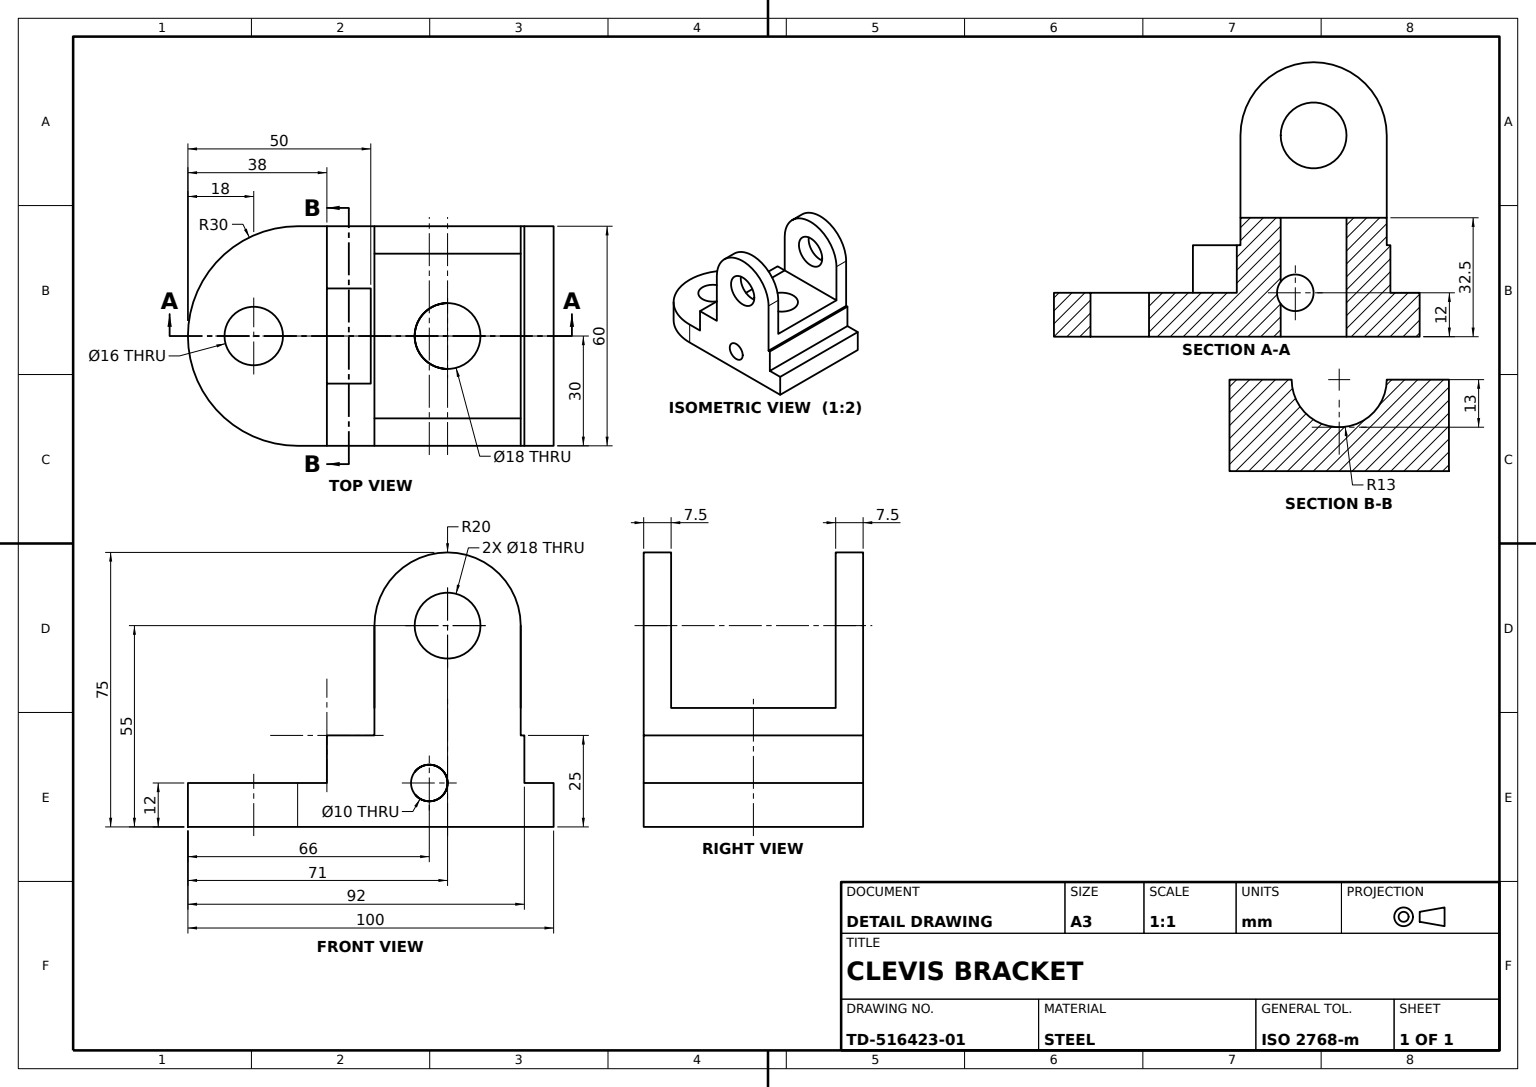
SolidWorks part; units mm, degrees
material "Plain Carbon Steel"
ref_plane "Front Plane" through (0, 0, 0) normal (0, 0, 1) x (1, 0, 0)
ref_plane "Top Plane" through (0, 0, 0) normal (0, 1, 0) x (1, 0, 0)
ref_plane "Right Plane" through (0, 0, 0) normal (1, 0, 0) x (0, 0, -1)
sketch "Base Plate Sketch" plane through (0, 0, 0) normal (0, 1, 0) x (1, 0, 0)
  line L0 (0, 0) -> (30, 0)
  line L1 (0, 0) -> (-30, 0)
  line L2 (-30, 0) -> (-30, 100)
  line L3 (-30, 100) -> (30, 100)
  line L4 (30, 100) -> (30, 0)
  dimension "D1" = 100
  dimension "D2" = 30
  dimension "D3" = 30
extrude "Base Plate" add sketch "Base Plate Sketch" along normal blind 12
sketch "Base Hole Sketch" plane through (0, 12, 0) normal (0, 1, 0) x (1, 0, 0)
  line L0 (-30, 30) -> (-30, 0)
  line L1 (-30, 0) -> (30, 0)
  line L2 (30, 0) -> (30, 30)
  circle A0 centre (0, 30) radius 30
  line M3 (-30, 0) -> (30, 0)
  line M4 (30, 0) -> (30, 100)
  line M6 (-30, 100) -> (-30, 0)
extrude "Base Hole" cut sketch "Base Hole Sketch" against normal blind 12 contours A0 M6 M3 | A0 L1 M4
sketch "Upright Block Sketch" plane through (30, 0, 0) normal (1, 0, 0) x (0, 0, -1)
  line L0 (100, 0) -> (50, 0)
  line L1 (30, 0) -> (100, 0) construction
  line L2 (50, 0) -> (50, 25)
  line L3 (50, 25) -> (62, 25)
  line L4 (62, 25) -> (92, 25)
  line L5 (92, 25) -> (92, 0)
  line L6 (30, 0) -> (30, 12) construction
  line M2 (30, 0) -> (100, 0)
  line M4 (100, 12) -> (30, 12)
  dimension "D1" = 20
  dimension "D2" = 32
  dimension "D3" = 62
  dimension "D4" = 25
extrude "Upright Block" add sketch "Upright Block Sketch" against normal blind 60 contours L5 L4 L3 L2 M4 | L5 L2 M4 M2
sketch "Clevis Ear Sketch" plane through (-30, 0, 0) normal (-1, 0, 0) x (0, 0, 1)
  line L0 (-50, 12) -> (-30, 12) construction
  line L1 (-50, 25) -> (-92, 25) construction
  line L2 (-51, 55) -> (-51, 25)
  line L3 (-51, 25) -> (-91, 25)
  line L4 (-91, 25) -> (-91, 55)
  arc A0 (-51, 55) -> (-91, 55) centre (-71, 55) ccw
  dimension "D1" = 20
  dimension "D2" = 41
  dimension "D3" = 43
extrude "Clevis Ear" add sketch "Clevis Ear Sketch" against normal blind 7.5
mirror "Clevis Ear Mirror" about plane through (0, 0, 0) normal (1, 0, 0) of "Clevis Ear"
sketch "Clevis Ear Extension Sketch" plane through (0, 25, 0) normal (0, 1, 0) x (1, 0, 0)
  line L0 (-22.5, 91) -> (-22.5, 51)
  line L1 (-22.5, 51) -> (22.5, 51)
  line L2 (22.5, 51) -> (22.5, 91)
  line L3 (22.5, 91) -> (-22.5, 91)
extrude "Clevis Ear Extension" add sketch "Clevis Ear Extension Sketch" along normal blind 7.5
sketch "Clevis Pin Bore Sketch" plane through (0, 32.5, 0) normal (0, 1, 0) x (1, 0, 0)
  line L0 (-22.5, 91) -> (-22.5, 51) construction
  line L1 (22.5, 91) -> (-22.5, 91) construction
  circle A0 centre (0, 71) radius 9
  dimension "D1" = 18
  dimension "D2" = 22.5
  dimension "D3" = 20
extrude "Clevis Pin Bore" cut sketch "Clevis Pin Bore Sketch" against normal blind 90.5
sketch "Saddle Block Sketch" plane through (30, 0, 0) normal (1, 0, 0) x (0, 0, -1)
  line L0 (50, 12) -> (38, 12)
  line L1 (30, 12) -> (50, 12) construction
  line L2 (38, 12) -> (38, 25)
  line L3 (38, 25) -> (50, 25)
  line L4 (50, 25) -> (50, 12)
  dimension "D1" = 62
extrude "Saddle Block" add sketch "Saddle Block Sketch" against normal blind 60
sketch "Saddle Cut Sketch" plane through (0, 0, -38) normal (0, 0, 1) x (1, 0, 0)
  line L0 (30, 25) -> (-30, 25) construction
  circle A0 centre (0, 25) radius 13
  dimension "D1" = 26
extrude "Saddle Cut" cut sketch "Saddle Cut Sketch" against normal blind 12
sketch "Through Hole A Sketch" plane through (-30, 0, 0) normal (-1, 0, 0) x (0, 0, 1)
  circle A0 centre (-71, 55) radius 9
  dimension "D1" = 18
extrude "Through Hole A" cut sketch "Through Hole A Sketch" against normal blind 139
sketch "Through Hole B Sketch" plane through (-30, 0, 0) normal (-1, 0, 0) x (0, 0, 1)
  circle A0 centre (-66, 12) radius 5
  dimension "D1" = 10
  dimension "D2" = 66
  dimension "D3" = 12
extrude "Through Hole B" cut sketch "Through Hole B Sketch" against normal blind 139
sketch "Through Hole C Sketch" plane through (0, 12, 0) normal (0, 1, 0) x (1, 0, 0)
  line L0 (30, 30) -> (30, 38) construction
  line L1 (-30, 38) -> (0, 38) construction
  circle A0 centre (0, 18) radius 8
  dimension "D1" = 16
  dimension "D2" = 30
  dimension "D3" = 20
extrude "Through Hole C" cut sketch "Through Hole C Sketch" against normal blind 139
